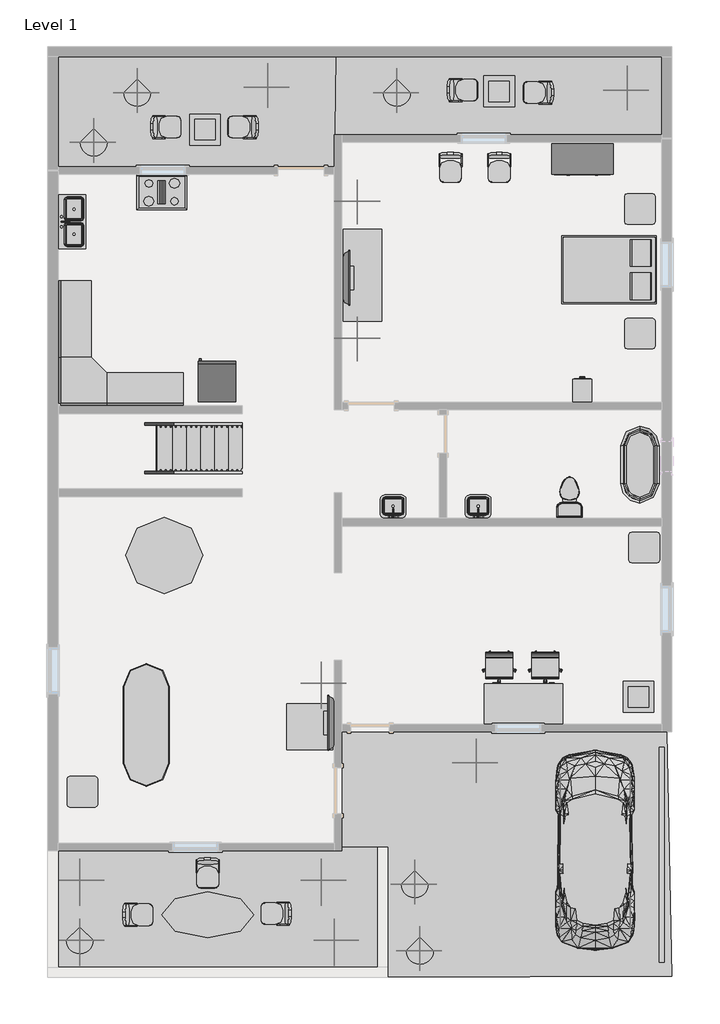
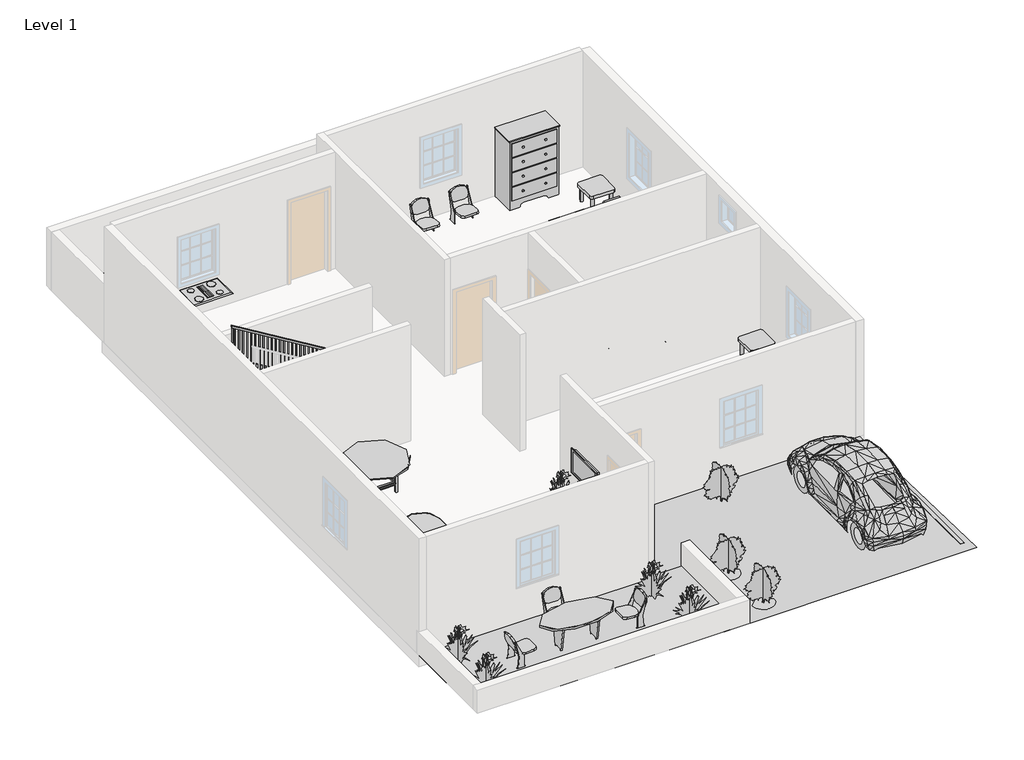
# One storey, part 2 of 2: 30 furniture elements, 15 geographic elements, 8 proxies, 6 flow terminals, 2 members, 1 railing, 1 stair flight.
# Revit data of these elements (continued)
# Materials (continued)
#   "Textile - Slate Blue": class "Fabric", colour RGB 98 102 118, transparency 0
#   "Laminate, Ivory, Matte": class "Plastic", colour RGB 247 247 239, transparency 0, Description = "Plastic Laminate - Ivory, Matte", Cost = 0
#   "Cherry": class "Wood", colour RGB 226 177 128, transparency 0, Description = "Prunus Serotina", Cost = 0
#   "Laminate - Ivory, Glossy": colour RGB 247 247 239, transparency 0
#   "Linen, Beige": class "Textile", colour RGB 249 239 230, transparency 0, Description = "Linen, beige", Cost = 0
#   "Steel, Paint Finish, Dark Gray, Matte": class "Metal", colour RGB 0 0 0, transparency 0, Description = "Steel, paint finish, dark gray, matte", Cost = 0
#   "Glass - Clear, Grey": class "Glass", colour RGB 252 255 255, transparency 0.64
#   "Pine": class "Wood", colour RGB 223 192 134, transparency 0, Description = "Pinus Echinata", Cost = 0
#   "Laminate - Black": colour RGB 0 0 0, transparency 0
#   "Textile - Light Gray": class "Fabric", colour RGB 204 204 204, transparency 0
#   "Parking Stripe": class "Paint", colour RGB 250 250 91, transparency 0
#   "TV - Black": colour RGB 49 49 49, transparency 0
#   "TV - Glass": colour RGB 157 157 157, transparency 0.9
#   "TV - Screen": colour RGB 0 0 0, transparency 0
